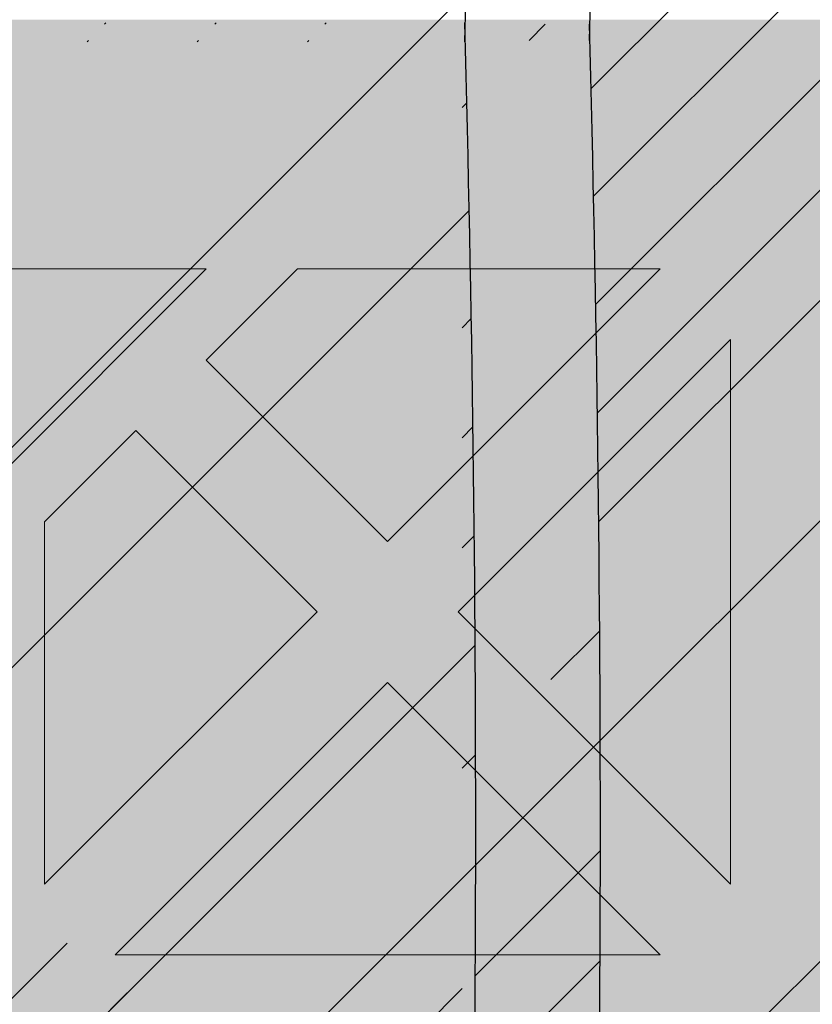
# Model space of a CAD drawing. Units: inches. Extents: x 844 to 2234, y 346 to 1084.
# Tile 11 of 93: x 1122.921 to 1124.948, y 693.702 to 696.22. Entities that reach past the tile are written whole.
import ezdxf

# ---------------------------------------------------------------- set-up
doc = ezdxf.new("R2010")
doc.units = ezdxf.units.IN
doc.header["$MEASUREMENT"] = 0
for name, color, linetype, lineweight in [('A-ANNO-DIMS', 2, 'Continuous', 18), ('furniture', 8, 'Continuous', 18), ('RA-AP-01$0$INT', 35, 'Continuous', 5)]:
    doc.layers.add(name, color=color, linetype=linetype, lineweight=lineweight)
doc.layers.add('RA-AP-01$0$FURN', color=3, linetype='Continuous')
doc.layers.add('RA-AP-01$0$WOOD', color=64, linetype='Continuous')
doc.styles.get("Standard").update_dxf_attribs({"font": 'arial.ttf'})
doc.dimstyles.get("Standard").update_dxf_attribs({"dimtxt": 6, "dimasz": 3, "dimexe": 0.18, "dimexo": 0.0625, "dimgap": 0.09, "dimtad": 0, "dimtih": 1, "dimtoh": 1, "dimdec": 1, "dimzin": 0, "dimdsep": 46, "dimlunit": 3, "dimtxsty": 'Standard', "dimblk": 'ARCHTICK', "dimcen": 0.09, "dimadec": 0, "dimazin": 0, "dimtfac": 1, "dimtdec": 1, "dimtofl": 0, "dimtmove": 0, "dimatfit": 3, "dimfxl": 1, "dimtolj": 1, "dimtzin": 0, "dimarcsym": 0})

# ---------------------------------------------------------------- blocks, each defined once
blk = doc.blocks.new('A$C18D01794')
at = {"layer": 'RA-AP-01$0$INT'}
h = blk.add_hatch(color=256, dxfattribs=at)
h.paths.add_polyline_path([(4.585917135068448, -6.356712009588273), (4.614201406330596, -6.356712009589021), (4.668846067270487, -6.411356670531338), (4.723490728212344, -6.356712009591912), (4.771774999457151, -6.35671200959319), (4.826419660396886, -6.411356670535356), (4.862780050090322, -6.374996280843536), (4.844495778842715, -6.356712009595112), (4.862780050090411, -6.356712009595595), (4.905206456960182, -6.399138416468211), (4.947632863832445, -6.356712009597838), (4.965917135079675, -6.356712009598322), (4.947632863831759, -6.374996280845421), (4.983993253523576, -6.411356670538857), (5.038637914464627, -6.356712009600247), (5.08692218571208, -6.356712009601523), (5.141566846649976, -6.411356670541852), (5.196211507589851, -6.356712009604411), (5.224495778822615, -6.356712009605161), (4.905206456953975, -6.676001331473793)])
h.paths.add_polyline_path([(4.895206456956031, -6.637717060225675), (4.895206456958921, -6.528427738347902), (4.840561796018589, -6.583072399285802)], flags=16)
h.paths.add_polyline_path([(4.915206456955638, -6.637717060226121), (4.969851117895509, -6.583072399288678), (4.915206456957609, -6.528427738348344)], flags=16)
h.paths.add_polyline_path([(4.826419660395175, -6.568930263661755), (4.881064321335613, -6.514285602723745), (4.771774999456703, -6.514285602720857)], flags=16)
h.paths.add_polyline_path([(4.983993253519558, -6.568930263665262), (5.038637914460456, -6.514285602726792), (4.929348592581548, -6.514285602724816)], flags=16)
h.paths.add_polyline_path([(4.881064321336025, -6.494285602723742), (4.826419660397532, -6.439640941782821), (4.771774999457062, -6.494285602720859)], flags=16)
h.paths.add_polyline_path([(4.929348592582019, -6.494285602724817), (5.038637914460982, -6.494285602726792), (4.983993253522945, -6.439640941786327)], flags=16)
h.paths.add_polyline_path([(4.895206456960191, -6.480143467100443), (4.895206456962115, -6.407422687715913), (4.876922185715016, -6.389138416467584), (4.840561796021581, -6.425498806159401)], flags=16)
h.paths.add_polyline_path([(4.915206456958487, -6.480143467100889), (4.969851117899527, -6.425498806162279), (4.933490728206909, -6.389138416468043), (4.9152064569598, -6.40742268771434)], flags=16)
h.paths.add_polyline_path([(4.757632863832376, -6.480143467096812), (4.812277524772842, -6.425498806158772), (4.757632863834348, -6.370854145217844)], flags=16)
h.paths.add_polyline_path([(4.737632863832376, -6.480143467096286), (4.737632863834348, -6.370854145217375), (4.682988202893906, -6.425498806155385)], flags=16)
h.paths.add_polyline_path([(5.05278005008503, -6.480143467103376), (5.052780050087917, -6.370854145224413), (4.998135389146995, -6.425498806162908)], flags=16)
h.paths.add_polyline_path([(5.072780050085024, -6.480143467103744), (5.127424711025931, -6.42549880616527), (5.072780050087916, -6.370854145224832)], flags=16)
h.paths.add_polyline_path([(4.935917135072783, -6.706712009592292), (5.255206456948811, -6.387422687716309), (5.255206456948932, -6.415706958964177), (5.200561796010279, -6.470351619902839), (5.255206456949403, -6.524996280841948), (5.25520645694961, -6.5732805520894), (5.200561796009787, -6.627925213029239), (5.236922185702417, -6.664285602721864), (5.255206456949919, -6.646001331474357), (5.255206456949998, -6.664285602721898), (5.212780050078687, -6.706712009592262), (5.25520645695036, -6.749138416463932), (5.255206456950438, -6.767422687711313), (5.236922185702424, -6.749138416463297), (5.200561796009796, -6.785498806155928), (5.255206456950753, -6.840143467096874), (5.25520645695096, -6.888427738341682), (5.200561796010322, -6.943072399282328), (5.255206456951428, -6.997717060223427), (5.255206456951547, -7.026001331471006)])
h.paths.add_polyline_path([(5.042988202883395, -6.785498806155427), (5.097632863823085, -6.840143467095101), (5.097632863822622, -6.730854145216193)], flags=16)
h.paths.add_polyline_path([(5.028846067259663, -6.771356670531693), (5.083490728198774, -6.716712009592573), (4.974201406321001, -6.716712009593042)], flags=16)
h.paths.add_polyline_path([(5.117632863823087, -6.840143467095186), (5.172277524762331, -6.785498806155926), (5.11763286382262, -6.730854145216225)], flags=16)
h.paths.add_polyline_path([(5.08349072819877, -6.696712009593886), (5.028846067259652, -6.642067348654775), (4.974201406320998, -6.696712009593438)], flags=16)
h.paths.add_polyline_path([(5.131774999446817, -6.854285602718917), (5.186419660386065, -6.799640941779662), (5.241064321325782, -6.854285602719365)], flags=17)
h.paths.add_polyline_path([(5.131774999446228, -6.716712009592374), (5.186419660386065, -6.771356670532194), (5.222780050079488, -6.734996280838764), (5.204495778832781, -6.716712009592063)], flags=16)
h.paths.add_polyline_path([(5.097632863822613, -6.682569873970264), (5.097632863823061, -6.573280552091354), (5.042988202883383, -6.627925213031044)], flags=16)
h.paths.add_polyline_path([(5.131774999446899, -6.874285602718915), (5.241064321325809, -6.874285602719364), (5.186419660386591, -6.928930263658598)], flags=17)
h.paths.add_polyline_path([(5.131774999446226, -6.696712009594078), (5.204495778830767, -6.696712009594374), (5.22278005007868, -6.67842773834687), (5.186419660386049, -6.642067348654249)], flags=16)
h.paths.add_polyline_path([(5.11763286382262, -6.682569873970225), (5.17227752476232, -6.627925213030515), (5.117632863823064, -6.573280552091267)], flags=16)
h.paths.add_polyline_path([(5.186419660386069, -6.613783077405491), (5.241064321325754, -6.559138416465795), (5.131774999446791, -6.559138416466263)], flags=16)
h.paths.add_polyline_path([(5.131774999446872, -6.539138416466263), (5.24106432132578, -6.539138416465794), (5.186419660386554, -6.484493755526573)], flags=16)
h.paths.add_polyline_path([(5.255206456951811, -7.08742268770861), (5.255206456951895, -7.106712009588038), (4.555206456956052, -7.106712009588038), (4.555206456956136, -7.087422687708617), (4.905206456953973, -6.737422687710788)])
h.paths.add_polyline_path([(4.983993253513404, -6.8444937555241), (4.92934859257295, -6.899138416462108), (5.03863791445186, -6.899138416465014)], flags=16)
h.paths.add_polyline_path([(4.969851117889988, -6.83035161990006), (4.915206456952556, -6.775706958960171), (4.915206456949648, -6.884996280837944)], flags=16)
h.paths.add_polyline_path([(4.929348592572535, -6.919138416462105), (4.983993253511019, -6.973783077403037), (5.038637914451496, -6.919138416465012)], flags=16)
h.paths.add_polyline_path([(5.052780050074912, -6.93328055208906), (4.998135389134438, -6.987925213027088), (5.052780050072919, -7.042569873968025)], flags=16)
h.paths.add_polyline_path([(5.07278005007491, -6.933280552089588), (5.072780050072918, -7.042569873968497), (5.127424711013374, -6.987925213030498)], flags=16)
h.paths.add_polyline_path([(4.89520645695295, -6.775706958959721), (4.840561796013067, -6.830351619897157), (4.895206456950961, -6.884996280837494)], flags=16)
h.paths.add_polyline_path([(4.915206456948365, -6.933280552085403), (4.915206456946434, -7.006001331471951), (4.933490728192729, -7.024285602719066), (4.969851117886972, -6.987925213026453)], flags=16)
h.paths.add_polyline_path([(4.881064321327021, -6.899138416461022), (4.82641966038902, -6.84449375552057), (4.771774999448108, -6.899138416459029)], flags=16)
h.paths.add_polyline_path([(4.895206456950073, -6.933280552084951), (4.840561796009022, -6.987925213023558), (4.876922185700835, -7.024285602716997), (4.895206456948749, -7.006001331469487)], flags=16)
h.paths.add_polyline_path([(4.983993253510392, -7.0020673486505), (4.947632863816944, -7.038427738342319), (4.965917135064043, -7.05671200959023), (5.038637914448995, -7.056712009591555)], flags=16)
h.paths.add_polyline_path([(4.881064321326543, -6.91913841646102), (4.771774999447578, -6.919138416459031), (4.826419660385607, -6.973783077399508)], flags=16)
h.paths.add_polyline_path([(4.905206456946447, -7.014285602717636), (4.862780050074785, -7.056712009588352), (4.947632863816685, -7.056712009589775)], flags=16)
h.paths.add_polyline_path([(5.14156684663679, -7.002067348654549), (5.086922185696452, -7.056712009592438), (5.196211507574223, -7.056712009594425)], flags=16)
h.paths.add_polyline_path([(4.8264196603837, -7.002067348646972), (4.771774999442643, -7.056712009585575), (4.8444957788276, -7.056712009587508), (4.862780050075511, -7.038427738340416)], flags=16)
h.paths.add_polyline_path([(4.812277524760289, -6.98792521302292), (4.757632863822258, -6.933280552082447), (4.757632863819352, -7.042569873961408)], flags=16)
h.paths.add_polyline_path([(4.73763286382226, -6.933280552082079), (4.682988202881349, -6.987925213020536), (4.737632863819352, -7.04256987396099)], flags=16)
h.paths.add_polyline_path([(4.723490728195188, -7.056712009584289), (4.668846067257299, -7.002067348643949), (4.614201406317417, -7.056712009581383)], flags=16)
h.paths.add_polyline_path([(4.597632863829262, -6.706712009592262), (4.555206456957951, -6.664285602721896), (4.555206456958029, -6.646001331474357), (4.573490728205535, -6.664285602721864), (4.609851117898167, -6.627925213029238), (4.555206456958338, -6.573280552089402), (4.555206456958546, -6.524996280841952), (4.60985111789767, -6.470351619902839), (4.555206456959015, -6.415706958964177), (4.555206456959138, -6.387422687716309), (4.874495778835167, -6.70671200959229), (4.5552064569564, -7.026001331471015), (4.555206456956523, -6.997717060223433), (4.609851117897629, -6.94307239928233), (4.555206456956988, -6.888427738341681), (4.555206456957198, -6.840143467096881), (4.609851117898153, -6.78549880615593), (4.573490728205528, -6.749138416463297), (4.555206456957507, -6.76742268771132), (4.555206456957585, -6.749138416463933)])
h.paths.add_polyline_path([(4.712780050085332, -6.730854145216195), (4.712780050084863, -6.840143467095105), (4.767424711024555, -6.785498806155427)], flags=16)
h.paths.add_polyline_path([(4.726922185709173, -6.716712009592573), (4.781566846648288, -6.771356670531693), (4.836211507586949, -6.716712009593043)], flags=16)
h.paths.add_polyline_path([(4.692780050085327, -6.730854145216225), (4.638135389145619, -6.785498806155928), (4.692780050084865, -6.840143467095185)], flags=16)
h.paths.add_polyline_path([(4.726922185709182, -6.696712009593886), (4.836211507586949, -6.696712009593436), (4.7815668466483, -6.642067348654773)], flags=16)
h.paths.add_polyline_path([(4.678637914461726, -6.71671200959237), (4.605917135075169, -6.716712009592063), (4.587632863828464, -6.734996280838766), (4.623993253521887, -6.771356670532195)], flags=16)
h.paths.add_polyline_path([(4.712780050085336, -6.68256987397026), (4.767424711024568, -6.627925213031042), (4.71278005008489, -6.573280552091352)], flags=16)
h.paths.add_polyline_path([(4.678637914461726, -6.696712009594076), (4.623993253521899, -6.642067348654247), (4.587632863829271, -6.67842773834687), (4.605917135077185, -6.696712009594376)], flags=16)
h.paths.add_polyline_path([(4.692780050085336, -6.682569873970228), (4.692780050084889, -6.573280552091267), (4.638135389145632, -6.627925213030515)], flags=16)
h.paths.add_polyline_path([(4.623993253521885, -6.799640941779662), (4.678637914461131, -6.854285602718915), (4.56934859258217, -6.854285602719365)], flags=17)
h.paths.add_polyline_path([(4.623993253521901, -6.613783077405509), (4.678637914461158, -6.559138416466263), (4.569348592582195, -6.559138416465795)], flags=16)
h.paths.add_polyline_path([(4.678637914461051, -6.874285602718915), (4.623993253521361, -6.928930263658598), (4.569348592582143, -6.874285602719364)], flags=17)
h.paths.add_polyline_path([(4.678637914461076, -6.539138416466263), (4.623993253521399, -6.484493755526573), (4.569348592582167, -6.539138416465796)], flags=16)
h = blk.add_hatch(color=256, dxfattribs=at)
h.paths.add_polyline_path([(4.895206456952951, -6.77570695895972), (4.840561796013068, -6.830351619897156), (4.895206456950958, -6.884996280837495)])
h.paths.add_polyline_path([(4.915206456949649, -6.884996280837942), (4.969851117889987, -6.830351619900054), (4.915206456952556, -6.775706958960171)])
h.paths.add_polyline_path([(5.038637914451862, -6.899138416465013), (4.983993253513403, -6.8444937555241), (4.929348592572953, -6.899138416462106)])
h.paths.add_polyline_path([(4.929348592572535, -6.919138416462105), (4.983993253511018, -6.973783077403037), (5.038637914451497, -6.919138416465012)])
h.paths.add_polyline_path([(4.915206456948366, -6.933280552085397), (4.915206456946433, -7.006001331471951), (4.93349072819273, -7.024285602719068), (4.969851117886972, -6.987925213026454)])
h.paths.add_polyline_path([(5.038637914448995, -7.056712009591553), (4.983993253510389, -7.002067348650502), (4.947632863816946, -7.038427738342318), (4.965917135064043, -7.05671200959023)])
h.paths.add_polyline_path([(5.05278005007292, -7.042569873968023), (5.05278005007491, -6.933280552089059), (4.998135389134438, -6.987925213027088)])
h.paths.add_polyline_path([(5.07278005007292, -7.042569873968496), (5.127424711013374, -6.987925213030498), (5.072780050074909, -6.933280552089588)])
h.paths.add_polyline_path([(5.141566846636789, -7.002067348654547), (5.086922185696449, -7.056712009592438), (5.196211507574223, -7.056712009594425)])
h.paths.add_polyline_path([(4.947632863816688, -7.056712009589774), (4.905206456946449, -7.014285602717634), (4.862780050074784, -7.056712009588353)])
h.paths.add_polyline_path([(4.840561796009025, -6.987925213023556), (4.876922185700834, -7.024285602716997), (4.895206456948747, -7.006001331469488), (4.895206456950075, -6.933280552084953)])
h.paths.add_polyline_path([(4.88106432132654, -6.919138416461021), (4.771774999447577, -6.919138416459031), (4.826419660385606, -6.973783077399508)])
h.paths.add_polyline_path([(4.881064321327019, -6.899138416461022), (4.826419660389019, -6.844493755520571), (4.771774999448108, -6.89913841645903)])
h.paths.add_polyline_path([(4.757632863819352, -7.042569873961409), (4.812277524760284, -6.987925213022922), (4.757632863822259, -6.933280552082447)])
h.paths.add_polyline_path([(4.8264196603837, -7.002067348646974), (4.771774999442646, -7.056712009585575), (4.844495778827599, -7.05671200958751), (4.862780050075512, -7.038427738340417)])
h.paths.add_polyline_path([(4.737632863819352, -7.042569873960988), (4.737632863822258, -6.933280552082078), (4.682988202881349, -6.987925213020538)])
h.paths.add_polyline_path([(4.668846067257299, -7.002067348643952), (4.61420140631742, -7.056712009581384), (4.723490728195189, -7.056712009584292)])
for p, q in [((5.038637914451498, -6.919138416465012), (4.929348592572535, -6.919138416462105)), ((4.929348592572535, -6.919138416462105), (4.983993253511019, -6.973783077403037)), ((5.038637914451498, -6.919138416465012), (4.983993253511019, -6.973783077403037)), ((4.915206456946434, -7.006001331470351), (4.915206456948367, -6.933280552085399)), ((4.915206456948367, -6.933280552085399), (4.969851117886972, -6.987925213026453)), ((5.05278005007491, -6.93328055208906), (4.998135389134438, -6.987925213027088)), ((5.05278005007491, -6.93328055208906), (5.052780050072921, -7.042569873968023)), ((4.969851117886972, -6.987925213026452), (4.93349072819353, -7.024285602718265)), ((5.052780050072921, -7.042569873968023), (4.998135389134438, -6.987925213027088)), ((4.98399325351039, -7.002067348650502), (4.947632863816946, -7.038427738342317)), ((5.038637914448995, -7.056712009591555), (4.983993253510388, -7.002067348650502)), ((4.915206456946427, -7.006001331471944), (4.933490728193524, -7.02428560271986)), ((4.905206456946449, -7.014285602717635), (4.94763286381669, -7.056712009589775)), ((4.947632863816946, -7.038427738342317), (4.965917135063997, -7.056712009590183)), ((4.965917135064043, -7.056712009590231), (4.947632863816944, -7.038427738342317)), ((4.94763286381669, -7.056712009589775), (4.862780050074783, -7.056712009588354)), ((4.965917135064043, -7.05671200959023), (5.038637914448995, -7.056712009591555))]:
    blk.add_line(p, q, dxfattribs=at)
blk = doc.blocks.new('A$C32926AE1')
at = {"layer": 'RA-AP-01$0$FURN'}
h = blk.add_hatch(dxfattribs=at)
h.set_pattern_fill('ANSI31', color=256, scale=0.1, style=0)
h.set_pattern_definition([(45, (0, 0), (-0.0088388347648318, 0.0088388347648318), [])])
edge = h.paths.add_edge_path(flags=16)
edge.add_arc((4.904771284329206, 4.246793130718756), 0.2603971832811541, 75.22398030683196, 104.7760196931204)
edge.add_arc((4.904771284329206, 4.246793130718756), 0.2603971832811541, 75.223980306832, 104.77601969312039, ccw=False)
edge = h.paths.add_edge_path(flags=16)
edge.add_arc((4.904771284329206, 4.067062675376612), 0.2603971832811541, 255.2239803068796, 284.776019693168)
edge.add_arc((4.904771284329206, 4.067062675376612), 0.2603971832811541, 255.22398030687958, 284.77601969316805, ccw=False)
edge = h.paths.add_edge_path(flags=0)
edge.add_arc((4.904771284329206, 4.067062675376612), 0.2603971832811541, 255.2239803068796, 284.776019693168)
edge.add_arc((4.904771284329206, 4.067062675376612), 0.2603971832811541, 255.22398030687958, 284.77601969316805, ccw=False)
edge = h.paths.add_edge_path(flags=0)
edge.add_arc((4.904771284329206, 4.067062675376612), 0.2603971832811541, 255.2239803068796, 284.776019693168)
edge.add_arc((4.904771284329206, 4.067062675376612), 0.2603971832811541, 255.22398030687958, 284.77601969316805, ccw=False)
edge = h.paths.add_edge_path()
edge.add_arc((4.604388392048174, 4.588829985554312), 0.1599999999999918, 342.3781640246255, 354.4317409793762)
edge.add_arc((5.090145208887507, 4.43216705527679), 0.3503971832811637, 162.0091218307731, 180.3186872093483)
edge.add_arc((5.205154176610243, 4.588829985554953), 0.1599999999999917, 185.5682590208461, 197.6218359767349)
edge.add_arc((4.904771284329229, 4.246793130718735), 0.3503971832811761, 72.00912183053516, 107.9908781690354)
edge.add_arc((9.535952835716557, 4.28682295566602), 4.798342501046485, 178.2875002453811, 181.5576802719453)
edge.add_arc((4.719397359771122, 4.43216705527679), 0.3503971832811637, 359.6813127906516, 377.9908781692269)
edge.add_arc((9.535967292294904, 4.286822350292874), 4.778371420254705, 178.2965938931842, 181.5667745797229)
edge.add_arc((4.719397359771122, 4.43216705527679), 0.3303971832811637, 359.6813127906516, 377.9908781692269)
edge.add_arc((0.2735752763637294, 4.286822350292874), 4.7783714202547, 358.4332254202771, 361.7034061068158)
edge.add_arc((5.061434214606998, 4.732549947558029), 0.1600000000000254, 252.3781640250584, 264.4317409792362)
edge.add_arc((4.748108354051257, 4.732549947558012), 0.1600000000000541, 275.5682590208426, 287.6218359759532)
edge.add_arc((4.604388392048115, 4.588829985554317), 0.1800000000000505, 342.3567572500182, 349.3735009646207)
edge.add_arc((5.205154176610254, 4.588829985554976), 0.1800000000000069, 190.6264990356027, 197.6432427513933)
edge.add_arc((5.061434214607106, 4.732549947558013), 0.1800000000000424, 252.3567572496606, 259.3735009644582)
edge.add_arc((4.904771284329208, 4.246793130718737), 0.3303971832811676, 71.99844483668534, 108.0015551637021)
edge.add_arc((4.748108354051414, 4.732549947558045), 0.1800000000000547, 280.6264990355479, 287.6432427495938)
edge.add_arc((5.090145208887514, 4.432167055276789), 0.2803971832811691, 162.8706300666893, 180.816523289902)
edge.add_arc((4.719397359771136, 4.432167055276689), 0.2803971832811534, 359.183476710103, 377.1293699333214)
edge.add_arc((4.904771284329222, 4.246793130718737), 0.2803971832811769, 72.87063006672916, 107.1293699332334)
edge.add_arc((5.090145208887522, 4.432167055276788), 0.2603971832811776, 165.2239803068007, 180.9953123810312)
edge.add_arc((4.719397359771141, 4.432167055276699), 0.2603971832811458, 359.0046876189768, 374.7760196932087)
edge.add_arc((5.090145208887507, 4.43216705527679), 0.3303971832811637, 162.0091218307731, 180.3186872093483)
edge.add_arc((9.53595427642584, 4.285015535491528), 4.728345371032053, 178.265043920078, 181.5679956281801)
edge.add_arc((0.2735882922327999, 4.285015535491582), 4.728345371032045, 358.4320043718193, 361.7349560799204)
edge.add_arc((9.535953591267507, 4.284458026472751), 4.708343996644348, 178.2573054306777, 181.5704995759608)
edge.add_arc((0.273588977391114, 4.284458026472785), 4.708343996644358, 358.4295004240388, 361.7426945693213)
edge.add_arc((0.2735889773911131, 4.029397779622582), 4.708343996644359, 358.2573054306787, 361.5704995759613)
edge.add_arc((9.535953591267518, 4.029397779622618), 4.708343996644359, 178.4295004240391, 181.7426945693223)
edge.add_arc((0.2735882922327901, 4.028840270603786), 4.728345371032054, 358.2650439200796, 361.5679956281808)
edge.add_arc((9.53595427642584, 4.028840270603841), 4.728345371032054, 178.4320043718199, 181.7349560799219)
edge.add_arc((0.2735752763637302, 4.027033455802493), 4.778371420254699, 358.2965938931842, 361.5667745797229)
edge.add_arc((4.719397359771122, 3.881688750818578), 0.3303971832811637, 342.0091218307731, 360.3186872093484)
edge.add_arc((5.090145208887507, 3.881688750818578), 0.3303971832811637, 179.6813127906516, 197.9908781692269)
edge.add_arc((9.535967292294904, 4.027033455802493), 4.778371420254705, 178.433225420277, 181.7034061068158)
edge.add_arc((4.719397359771122, 3.881688750818578), 0.3503971832811637, 342.0091218307731, 360.3186872093484)
edge.add_arc((9.53595283571655, 4.027032850429349), 4.79834250104648, 178.4423197280546, 181.7124997546188)
edge.add_arc((4.719397359771141, 3.881688750818669), 0.2603971832811458, 345.2239803067913, 360.9953123810232)
edge.add_arc((5.090145208887522, 3.88168875081858), 0.2603971832811776, 179.0046876189687, 194.7760196931993)
edge.add_arc((4.904771284329222, 4.067062675376631), 0.2803971832811769, 252.8706300667665, 287.1293699332708)
edge.add_arc((4.719397359771136, 3.881688750818678), 0.2803971832811534, 342.8706300666787, 360.8165232898969)
edge.add_arc((5.090145208887514, 3.881688750818579), 0.2803971832811691, 179.183476710098, 197.1293699333106)
edge.add_arc((4.748108354051414, 3.581305858537323), 0.1800000000000547, 72.3567572504062, 79.37350096445199)
edge.add_arc((4.904771284329208, 4.067062675376631), 0.3303971832811676, 251.9984448362979, 288.0015551633146)
edge.add_arc((5.061434214607106, 3.581305858537355), 0.1800000000000424, 100.6264990355418, 107.6432427503394)
edge.add_arc((5.205154176610254, 3.725025820540392), 0.1800000000000069, 162.3567572486066, 169.3735009643972)
edge.add_arc((4.604388392048115, 3.725025820541051), 0.1800000000000505, 10.62649903537925, 17.64324274998182)
edge.add_arc((4.748108354051257, 3.581305858537356), 0.1600000000000541, 72.37816402404681, 84.43174097915735)
edge.add_arc((4.904771284329229, 4.067062675376632), 0.3503971832811761, 252.0091218309645, 287.9908781694648)
edge.add_arc((5.061434214606998, 3.581305858537339), 0.1600000000000254, 95.56825902076373, 107.6218359749416)
edge.add_arc((5.205154176610243, 3.725025820540414), 0.1599999999999917, 162.3781640232651, 174.4317409791539)
edge.add_arc((5.090145208887507, 3.881688750818578), 0.3503971832811637, 179.6813127906516, 197.9908781692269)
edge.add_arc((4.604388392048174, 3.725025820541056), 0.1599999999999918, 5.568259020623824, 17.62183597537444)
edge.add_arc((0.2735897329420762, 4.28682295566602), 4.798342501046482, 358.4423197280547, 361.7124997546188)
edge.add_arc((0.2735897329420691, 4.027032850429348), 4.798342501046489, 358.2875002453812, 361.5576802719453)
at = {"layer": 'RA-AP-01$0$WOOD'}
h = blk.add_hatch(color=256, dxfattribs=at)
h.dxf.hatch_style = 1
h.paths.add_polyline_path([(5.157430609644524, 4.573483066760929, -0.1009492694046607), (5.155401577623758, 4.593365984175333, -0.1842662638101597), (5.172249623284174, 4.638795604568598, 0.2056608120311276), (5.179560981299304, 4.661316324430096, 0.3614336704623542), (5.134352340494423, 4.706524965234944, 0.2056608120311297), (5.111831620632933, 4.699213607219793, -0.1842662638101113), (5.066402000239693, 4.682365561559342, -0.1055311479399994), (5.045656153913092, 4.68467289944697, 0.1567636581983829), (4.763886414745334, 4.684672899446966, -0.1055311479399895), (4.743140568418733, 4.68236556155934, -0.1842662638100833), (4.6977109480255, 4.69921360721979, 0.2056608120302612), (4.675190228164109, 4.706524965234949, 0.3614336704708441), (4.629981587358889, 4.66131632442871, 0.2056608120245944), (4.637292945374126, 4.638795604567974, -0.1842662638101024), (4.654140991034615, 4.59336598417475, -0.1009492694055169), (4.652111959013835, 4.573483066760181, 0.021410119221476), (4.629748025606143, 4.156712009541676, 0.0214101192214795), (4.652111959013809, 3.739940952323101, -0.1009492694059586), (4.654140991034615, 3.720058034908448, -0.1842662638100975), (4.637292945374126, 3.674628414515226, 0.2056608120245705), (4.629981587358889, 3.652107694654492, 0.3614336704708879), (4.675190228164113, 3.606899053848249, 0.2056608120302384), (4.697710948025501, 3.614210411863408, -0.1842662638100995), (4.743140568418738, 3.63105845752386, -0.1055311479402541), (4.763886414745388, 3.628751119636215, 0.1567636581983776), (5.045656153913137, 3.628751119636244, -0.1055311479397538), (5.066402000239692, 3.631058457523857, -0.1842662638101067), (5.111831620632931, 3.614210411863407, 0.2056608120310924), (5.134352340494417, 3.606899053848256, 0.3614336704624001), (5.179560981299307, 3.652107694653103, 0.2056608120311314), (5.172249623284175, 3.6746284145146, -0.1842662638101402), (5.155401577623758, 3.72005803490786, -0.1009492694051366), (5.15743060964455, 3.739940952322354, 0.0214101192215073), (5.179794543052287, 4.156712009541468, 0.0214101192215252)])
h.paths.add_polyline_path([(4.639748609479751, 4.156712009541513, 0.0213537860821624), (4.661970494867118, 3.741887061152232, -0.094075836301374), (4.664143710413708, 3.7196126951003, -0.1824818158568985), (4.644813765429836, 3.668037719127816, 0.2056608120245319), (4.639939526753007, 3.653023905887301, 0.3614336704710246), (4.676106439397173, 3.616856993242342, 0.2056608120302234), (4.691120252638095, 3.621731231919122, -0.1824818158602558), (4.742695228611606, 3.641061176902986, -0.1029891339458722), (4.766991894714349, 3.638256818950944, 0.156709409989566), (5.042550673941472, 3.638256818950105, -0.102989133958497), (5.066847340047078, 3.641061176902949, -0.1824818158594995), (5.118422316020358, 3.621731231919103, 0.2056608120311416), (5.133436129261316, 3.616856993242346, 0.3614336704621468), (5.169603041905217, 3.653023905886178, 0.2056608120310986), (5.164728803228477, 3.668037719127177, -0.1824818158565612), (5.145398858244737, 3.719612695099578, -0.0940758363009313), (5.147572073791232, 3.741887061151398, 0.0213537860822023), (5.169793959178681, 4.156712009541451, 0.0213537860822226), (5.147572073791203, 4.571536957931898, -0.0940758363005034), (5.145398858244737, 4.59381132398362, -0.1824818158565587), (5.164728803228476, 4.645386299956021, 0.2056608120311045), (5.169603041905216, 4.66040011319702, 0.3614336704621845), (5.133436129261313, 4.696567025840856, 0.2056608120310773), (5.118422316020359, 4.691692787164098, -0.182481815859508), (5.066847340047078, 4.67236284218025, -0.1029891339584606), (5.04255067394148, 4.675167200133092, 0.156709409989566), (4.766991894714357, 4.675167200132257, -0.1029891339458842), (4.742695228611611, 4.672362842180213, -0.1824818158602725), (4.691120252638095, 4.691692787164077, 0.2056608120302152), (4.676106439397174, 4.696567025840858, 0.3614336704710363), (4.639939526753005, 4.660400113195899, 0.2056608120245495), (4.644813765429837, 4.645386299955384, -0.1824818158568934), (4.664143710413708, 4.593811323982902, -0.0940758363009187), (4.661970494867149, 4.571536957931074, 0.021353786082177)], flags=16)
h.paths.add_polyline_path([(5.129794543052235, 4.432167055276933, -0.0141661062790638), (5.130152669293814, 4.156927903047693, -0.0141661062790647), (5.129794543052234, 3.881688750818433, -0.0785247771143638), (5.10979738006795, 3.755143611847103, 0.0945969212073497), (5.105408519571111, 3.717898134952927, 0.1043170707844957), (5.116074640131521, 3.670385395016088, 0.1043170707864965), (5.068561900193738, 3.681051515576561, 0.09459692119553), (5.031316423304057, 3.676662655080835, -0.1580239521427272), (4.778226145355827, 3.676662655080367, 0.0945969211986668), (4.740980668464973, 3.681051515576592, 0.1043170707882822), (4.693467928526415, 3.670385395015844, 0.1043170707867916), (4.704134049087309, 3.717898134953662, 0.0945969211972894), (4.69974518859162, 3.755143611844042, -0.0785247771163196), (4.679748025606343, 3.881688750818406, -0.0141661062790663), (4.679389899364763, 4.156927903047693, -0.0141661062790672), (4.679748025606343, 4.432167055276998, -0.0785247771163064), (4.699745188591625, 4.55871219425134, 0.094596921197333), (4.704134049087308, 4.595957671141738, 0.1043170707867205), (4.693467928526416, 4.643470411079523, 0.1043170707882628), (4.740980668464965, 4.632804290518776, 0.0945969211988114), (4.778226145355874, 4.637193151015016, -0.158023952142669), (5.031316423304015, 4.637193151014546, 0.0945969211956361), (5.068561900193736, 4.632804290518806, 0.1043170707864979), (5.11607464013152, 4.643470411079278, 0.1043170707844617), (5.105408519571112, 4.595957671142455, 0.0945969212074597), (5.109797380067959, 4.558712194248236, -0.0785247771143467)], flags=0)
h.paths.add_polyline_path([(5.119794532311105, 4.432259799204851, -0.0142000800617244), (5.120156169157484, 4.156927903047701, -0.0142000800617277), (5.119794532311105, 3.881596006890482, -0.0784894509520253), (5.100273383573699, 3.758192358677797, 0.0940138827242913), (5.095413455884425, 3.717477693979438, 0.0606271852308753), (5.099615656341024, 3.686844378806616, 0.0606271852322524), (5.068982341167493, 3.691046579263239, 0.0940138827010453), (5.028267676478798, 3.686186651576848, -0.1580706864508061), (4.781274892180912, 3.686186651576435, 0.0940138827026903), (4.740560227491556, 3.691046579263279, 0.0606271852339895), (4.709926912317155, 3.686844378806508, 0.0606271852329405), (4.714129112773991, 3.717477693980356, 0.094013882701304), (4.709269185087677, 3.758192358669163, -0.0784894509577193), (4.689748036347473, 3.881596006890469, -0.014200080061729), (4.689386399501094, 4.156927903047709, -0.0142000800617217), (4.689748036347473, 4.432259799204808, -0.078489450957724), (4.709269185087651, 4.555663447426125, 0.0940138827014585), (4.714129112773992, 4.596378112114996, 0.0606271852329731), (4.709926912317154, 4.62701142728886, 0.0606271852340196), (4.74056022749157, 4.622809226832087, 0.0940138827024997), (4.781274892180847, 4.627669154518912, -0.1580706864508359), (5.028267676478777, 4.627669154518526, 0.0940138827010946), (5.068982341167492, 4.622809226832129, 0.060627185232254), (5.099615656341024, 4.627011427288751, 0.0606271852308727), (5.095413455884425, 4.59637811211593, 0.0940138827241088), (5.100273383573675, 4.555663447417647, -0.0784894509520978)], flags=0)
h.paths.add_polyline_path([(5.06978912287499, 4.430218106756144, -0.014241683694547), (5.070173729147532, 4.156927903047672, -0.0142416836945458), (5.06978912287499, 3.883637699339223, -0.0800609523125196), (5.052662118612511, 3.773463122773442, 0.0526421978001116), (5.04590916754064, 3.740550867606997, 0.0526421977992423), (5.012996912374707, 3.73379791653534, -0.1583028414718258), (4.796545656286308, 3.73379791653451, 0.0526421978034211), (4.763633401117837, 3.740550867607021, 0.0526421978018622), (4.756880450045755, 3.773463122774558, -0.0800609523117106), (4.739753445783639, 3.883637699339268, -0.0142416836945435), (4.739368839511098, 4.156927903047671, -0.0142416836945477), (4.739753445783639, 4.430218106756155, -0.0800609523116345), (4.75688045004574, 4.540392683320762, 0.052642197801941), (4.763633401117837, 4.573304938488346, 0.0526421978035071), (4.796545656286361, 4.580057889560873, -0.1583028414717561), (5.012996912374669, 4.580057889560039, 0.0526421977993048), (5.04590916754064, 4.57330493848837, 0.0526421978002057), (5.052662118612529, 4.540392683321868, -0.080060952312477)], flags=0)
h.paths.add_polyline_path([(5.049789715110557, 4.43038092723357, -0.0143097550741839), (5.05018085590259, 4.156927903047715, -0.0143097550741854), (5.049789715110558, 3.883474878861827, -0.0800685599149176), (5.03362098255317, 3.779581877367999, 0.0306258898956367), (5.028241146483733, 3.758218888663947, 0.0306258898977031), (5.006878157778253, 3.75283905259408, -0.1583983521624096), (4.802664410878162, 3.752839052594731, 0.0306258898946014), (4.781301422174808, 3.758218888663924, 0.0306258898967912), (4.775921586105202, 3.779581877368794, -0.080068559914251), (4.759752853548071, 3.883474878861786, -0.0143097550741854), (4.759361712756037, 4.156927903047671, -0.0143097550741854), (4.759752853548071, 4.430380927233557, -0.0800685599142479), (4.775921586105193, 4.534273928726546, 0.0306258898968306), (4.781301422174808, 4.555636917431444, 0.0306258898945754), (4.802664410878143, 4.561016753500631, -0.1583983521624168), (5.006878157778244, 4.561016753501291, 0.0306258898977177), (5.028241146483733, 4.555636917431421, 0.0306258898958182), (5.03362098255321, 4.534273928727244, -0.080068559914796)], flags=0)
h.paths.add_polyline_path([(4.999766070382627, 4.428171244713864, -0.0143443147609634), (5.000198441819402, 4.156927903047689, -0.0143443147609612), (4.999766070382627, 3.885684561381556, -0.0784641635803329), (4.987356730658798, 3.799103304488872, -0.1506053783831347), (4.822185837999821, 3.79910330448882, -0.0784641635803318), (4.809776498276007, 3.885684561381509, -0.014344314760963), (4.809344126839227, 4.156927903047677, -0.0143443147609645), (4.809776498276007, 4.428171244713873, -0.0784641635803192), (4.822185837999822, 4.514752501606549, -0.1506053783831338), (4.987356730658798, 4.514752501606494, -0.078464163580285)], flags=0)
h.paths.add_polyline_path([(4.979755254238824, 4.42764379880488, -0.0143772539198268), (4.980205517789977, 4.156927903047693, -0.0143772539198275), (4.979755254238824, 3.886212007290489, -0.0689242507424422), (4.971183264704897, 3.815276770442801, -0.1296645318904179), (4.838359303953726, 3.815276770442746, -0.0689242507424186), (4.829787314419809, 3.886212007290419, -0.0143772539198292), (4.829337050868653, 4.156927903047653, -0.0143772539198325), (4.829787314419809, 4.427643798804946, -0.0689242507424211), (4.838359303953725, 4.498579035652621, -0.1296645318904187), (4.971183264704897, 4.498579035652565, -0.0689242507424401)], flags=0)
h = blk.add_hatch(color=256, dxfattribs=at)
h.dxf.hatch_style = 1
h.paths.add_polyline_path([(5.145398858244737, 4.59381132398362, -0.1824818158565616), (5.164728803228476, 4.645386299956021, 0.2056608120311045), (5.169603041905216, 4.66040011319702, 0.3614336704621845), (5.133436129261313, 4.696567025840856, 0.2056608120310773), (5.118422316020359, 4.691692787164098, -0.182481815859508), (5.066847340047078, 4.67236284218025, -0.1029891339584606), (5.04255067394148, 4.675167200133092, 0.156709409989566), (4.766991894714357, 4.675167200132257, -0.1029891339458842), (4.742695228611611, 4.672362842180213, -0.1824818158602725), (4.691120252638095, 4.691692787164077, 0.2056608120302152), (4.676106439397174, 4.696567025840858, 0.3614336704710363), (4.639939526753005, 4.660400113195899, 0.2056608120245495), (4.644813765429837, 4.645386299955384, -0.1824818158568934), (4.664143710413708, 4.593811323982902, -0.0940758363009187), (4.661970494867149, 4.571536957931074, 0.0213537860821772), (4.639748609479751, 4.156712009541507, 0.0213537860821625), (4.661970494867119, 3.741887061152226, -0.0940758363013071), (4.664143710413708, 3.719612695100309, -0.1824818158569294), (4.644813765429836, 3.668037719127816, 0.2056608120245319), (4.639939526753007, 3.653023905887301, 0.3614336704710246), (4.676106439397173, 3.616856993242342, 0.2056608120302234), (4.691120252638095, 3.621731231919122, -0.1824818158602558), (4.742695228611606, 3.641061176902986, -0.1029891339458722), (4.766991894714349, 3.638256818950944, 0.156709409989566), (5.042550673941472, 3.638256818950105, -0.102989133958497), (5.066847340047078, 3.641061176902949, -0.1824818158594995), (5.118422316020358, 3.621731231919103, 0.2056608120311416), (5.133436129261316, 3.616856993242346, 0.3614336704621468), (5.169603041905217, 3.653023905886178, 0.2056608120310986), (5.164728803228477, 3.668037719127177, -0.1824818158565612), (5.145398858244737, 3.719612695099578, -0.0940758363009313), (5.147572073791232, 3.741887061151398, 0.0213537860822023), (5.169793959178681, 4.156712009541451, 0.0213537860822226), (5.147572073791203, 4.571536957931898, -0.0940758363004996)])
h.paths.add_polyline_path([(5.109797380067958, 4.55871219424824, -0.0785247771143472), (5.129794543052234, 4.432167055276936, -0.0141661062790644), (5.130152669293814, 4.156927903047685, -0.014166106279066), (5.129794543052234, 3.881688750818401, -0.0785247771143517), (5.109797380067946, 3.755143611847092, 0.0945969212073132), (5.105408519571111, 3.717898134952929, 0.1043170707844995), (5.116074640131521, 3.670385395016088, 0.1043170707864965), (5.068561900193738, 3.681051515576561, 0.09459692119553), (5.031316423304057, 3.676662655080835, -0.1580239521427272), (4.778226145355827, 3.676662655080367, 0.0945969211986668), (4.740980668464973, 3.681051515576592, 0.1043170707882822), (4.693467928526415, 3.670385395015844, 0.1043170707867916), (4.704134049087309, 3.717898134953662, 0.0945969211972894), (4.69974518859162, 3.755143611844042, -0.0785247771163196), (4.679748025606343, 3.881688750818406, -0.0141661062790663), (4.679389899364763, 4.156927903047693, -0.0141661062790672), (4.679748025606343, 4.432167055276998, -0.0785247771163064), (4.699745188591625, 4.55871219425134, 0.094596921197333), (4.704134049087308, 4.595957671141738, 0.1043170707867205), (4.693467928526416, 4.643470411079523, 0.1043170707882628), (4.740980668464965, 4.632804290518776, 0.0945969211988114), (4.778226145355874, 4.637193151015016, -0.158023952142669), (5.031316423304015, 4.637193151014546, 0.0945969211956361), (5.068561900193736, 4.632804290518806, 0.1043170707864979), (5.11607464013152, 4.643470411079278, 0.1043170707844617), (5.105408519571112, 4.595957671142455, 0.0945969212074504)], flags=16)
h.paths.add_polyline_path([(5.100273383573655, 4.55566344741771, -0.0784894509521388), (5.119794532311105, 4.432259799204852, -0.0142000800617252), (5.120156169157484, 4.156927903047686, -0.014200080061726), (5.119794532311105, 3.881596006890502, -0.0784894509520446), (5.100273383573696, 3.758192358677786, 0.0940138827242721), (5.095413455884425, 3.717477693979436, 0.0606271852308692), (5.099615656341024, 3.686844378806616, 0.0606271852322522), (5.068982341167493, 3.691046579263239, 0.0940138827010453), (5.028267676478798, 3.686186651576848, -0.1580706864508061), (4.781274892180912, 3.686186651576435, 0.0940138827026903), (4.740560227491556, 3.691046579263279, 0.0606271852339895), (4.709926912317155, 3.686844378806508, 0.0606271852329405), (4.714129112773991, 3.717477693980356, 0.094013882701304), (4.709269185087677, 3.758192358669163, -0.0784894509577193), (4.689748036347473, 3.881596006890469, -0.014200080061729), (4.689386399501094, 4.156927903047709, -0.0142000800617217), (4.689748036347473, 4.432259799204808, -0.078489450957724), (4.709269185087651, 4.555663447426125, 0.0940138827014585), (4.714129112773992, 4.596378112114996, 0.0606271852329731), (4.709926912317154, 4.62701142728886, 0.0606271852340196), (4.74056022749157, 4.622809226832087, 0.0940138827024997), (4.781274892180847, 4.627669154518912, -0.1580706864508359), (5.028267676478777, 4.627669154518526, 0.0940138827010946), (5.068982341167492, 4.622809226832129, 0.060627185232254), (5.099615656341024, 4.627011427288751, 0.0606271852308727), (5.095413455884425, 4.59637811211593, 0.094013882723957)], flags=0)
h.paths.add_polyline_path([(5.04590916754064, 4.57330493848837, 0.0526421978002057), (5.052662118612529, 4.540392683321868, -0.0800609523124783), (5.06978912287499, 4.430218106756142, -0.0142416836945469), (5.070173729147532, 4.156927903047672, -0.0142416836945458), (5.06978912287499, 3.883637699339223, -0.0800609523125196), (5.052662118612511, 3.773463122773442, 0.0526421978001116), (5.04590916754064, 3.740550867606997, 0.0526421977992423), (5.012996912374707, 3.73379791653534, -0.1583028414718258), (4.796545656286308, 3.73379791653451, 0.0526421978034211), (4.763633401117837, 3.740550867607021, 0.0526421978018622), (4.756880450045755, 3.773463122774558, -0.0800609523117106), (4.739753445783639, 3.883637699339268, -0.0142416836945435), (4.739368839511098, 4.156927903047671, -0.0142416836945477), (4.739753445783639, 4.430218106756155, -0.0800609523116345), (4.75688045004574, 4.540392683320762, 0.052642197801941), (4.763633401117837, 4.573304938488346, 0.0526421978035071), (4.796545656286361, 4.580057889560873, -0.1583028414717561), (5.012996912374669, 4.580057889560039, 0.0526421977993048)], flags=0)
h.paths.add_polyline_path([(5.028241146483733, 4.555636917431422, 0.0306258898956949), (5.033620982553182, 4.534273928727329, -0.0800685599148649), (5.049789715110557, 4.430380927233569, -0.0143097550741839), (5.05018085590259, 4.156927903047715, -0.0143097550741854), (5.049789715110558, 3.883474878861827, -0.0800685599149176), (5.03362098255317, 3.779581877367999, 0.0306258898956367), (5.028241146483733, 3.758218888663947, 0.0306258898977031), (5.006878157778253, 3.75283905259408, -0.1583983521624096), (4.802664410878162, 3.752839052594731, 0.0306258898946014), (4.781301422174808, 3.758218888663924, 0.0306258898967912), (4.775921586105202, 3.779581877368794, -0.080068559914251), (4.759752853548071, 3.883474878861786, -0.0143097550741854), (4.759361712756037, 4.156927903047671, -0.0143097550741854), (4.759752853548071, 4.430380927233557, -0.0800685599142479), (4.775921586105193, 4.534273928726546, 0.0306258898968306), (4.781301422174808, 4.555636917431444, 0.0306258898945754), (4.802664410878143, 4.561016753500631, -0.1583983521624168), (5.006878157778244, 4.561016753501291, 0.0306258898977174)], flags=0)
h.paths.add_polyline_path([(4.987356730658798, 4.514752501606494, -0.0784641635803018), (4.999766070382627, 4.428171244713845, -0.0143443147609637), (5.000198441819402, 4.156927903047665, -0.0143443147609622), (4.999766070382628, 3.885684561381514, -0.0784641635802952), (4.987356730658797, 3.799103304488872, -0.1506053783831338), (4.822185837999821, 3.799103304488819, -0.0784641635803342), (4.809776498276007, 3.885684561381512, -0.0143443147609628), (4.809344126839227, 4.156927903047676, -0.0143443147609646), (4.809776498276007, 4.428171244713873, -0.0784641635803192), (4.822185837999822, 4.514752501606549, -0.1506053783831338)], flags=0)
h.paths.add_polyline_path([(4.971183264704897, 4.498579035652566, -0.0689242507424384), (4.979755254238824, 4.427643798804883, -0.0143772539198276), (4.980205517789977, 4.15692790304768, -0.0143772539198258), (4.979755254238823, 3.88621200729051, -0.0689242507424628), (4.971183264704897, 3.815276770442801, -0.129664531890417), (4.838359303953726, 3.815276770442746, -0.0689242507424186), (4.829787314419809, 3.886212007290419, -0.0143772539198292), (4.829337050868653, 4.156927903047653, -0.0143772539198325), (4.829787314419809, 4.427643798804946, -0.0689242507424211), (4.838359303953725, 4.498579035652621, -0.1296645318904187)], flags=0)
h = blk.add_hatch(dxfattribs=at)
h.set_pattern_fill('ANSI31', color=256, scale=0.05, style=0)
h.set_pattern_definition([(45, (0, 0), (-0.0044194173824159, 0.0044194173824159), [])])
h.paths.add_polyline_path([(5.130152669293814, 4.156927903047704, 0.0141661062790657), (5.129794543052234, 4.432167055276982, 0.0777827904001433), (5.110168979996553, 4.557559993161921, -0.0976515123401879), (5.105408519571111, 4.595957671142454, -0.1043170707844687), (5.116074640131522, 4.64347041107928), (5.099615656341024, 4.627011427288751, 0.0606271852308727), (5.095413455884425, 4.59637811211593, 0.0940138827241088), (5.100273383573675, 4.555663447417647, -0.0784894509520972), (5.119794532311105, 4.432259799204852, -0.0142000800617252), (5.120156169157484, 4.156927903047686, -0.014200080061726), (5.119794532311105, 3.881596006890502, -0.0784894509520446), (5.100273383573696, 3.758192358677786, 0.0940138827242721), (5.095413455884425, 3.717477693979436, 0.0606271852308692), (5.099615656341024, 3.686844378806616), (5.116074640131519, 3.67038539501609, -0.1043170707844594), (5.105408519571112, 3.717898134952912, -0.0976515123401594), (5.11016897999655, 3.756295812933435, 0.0777827904001654), (5.129794543052234, 3.881688750818409, 0.0141661062790665)])
h.paths.add_polyline_path([(5.030164222210597, 3.676291055149937, -0.0976515123472002), (5.068561900193739, 3.681051515576561, -0.1043170707864927), (5.116074640131521, 3.670385395016088), (5.099615656341024, 3.686844378806616, 0.0606271852322522), (5.068982341167493, 3.691046579263239, 0.0940138827010453), (5.028267676478798, 3.686186651576848, -0.1580706864508061), (4.781274892180912, 3.686186651576435, 0.0940138827026903), (4.740560227491556, 3.691046579263279, 0.0606271852339913), (4.709926912317154, 3.686844378806508), (4.693467928526416, 3.670385395015845, -0.1043170707882796), (4.740980668464973, 3.681051515576592, -0.0976515123427246), (4.779378346446416, 3.676291055150394, 0.156512506893803)])
h.paths.add_polyline_path([(4.689748036347473, 3.881596006890472, -0.014200080061729), (4.689386399501094, 4.156927903047712, -0.0142000800617195), (4.689748036347473, 4.432259799204768, -0.078489450957742), (4.709269185087648, 4.555663447426114, 0.0940138827014821), (4.714129112773992, 4.596378112114995, 0.0606271852329748), (4.709926912317154, 4.62701142728886), (4.693467928526414, 4.643470411079524, -0.1043170707867939), (4.704134049087309, 4.595957671141706, -0.09765151234893), (4.699373588660725, 4.557559993157876, 0.0777827903975372), (4.679748025606343, 4.432167055276987, 0.0141661062790675), (4.679389899364763, 4.156927903047675, 0.0141661062790641), (4.679748025606343, 3.88168875081843, 0.0777827903975637), (4.699373588660724, 3.756295812937497, -0.0976515123490278), (4.704134049087308, 3.717898134953629, -0.1043170707867196), (4.693467928526416, 3.670385395015845), (4.709926912317155, 3.686844378806508, 0.0606271852329413), (4.714129112773991, 3.717477693980357, 0.0940138827013084), (4.709269185087676, 3.758192358669166, -0.0784894509577192)])
h.paths.add_polyline_path([(4.779378346446434, 4.63756475094498, -0.0976515123427943), (4.740980668464964, 4.632804290518776, -0.1043170707882609), (4.693467928526416, 4.643470411079523), (4.709926912317154, 4.62701142728886, 0.0606271852340196), (4.74056022749157, 4.622809226832087, 0.0940138827024997), (4.781274892180847, 4.627669154518912, -0.1580706864508359), (5.028267676478777, 4.627669154518526, 0.0940138827010946), (5.068982341167492, 4.622809226832129, 0.060627185232254), (5.099615656341024, 4.627011427288751), (5.116074640131521, 4.643470411079279, -0.1043170707865022), (5.068561900193735, 4.632804290518806, -0.0976515123475899), (5.030164222210446, 4.637564750945479, 0.1565125068936924)])
h = blk.add_hatch(dxfattribs=at)
h.set_pattern_fill('ANSI32', color=256, scale=0.2, style=0)
h.set_pattern_definition([(45, (0, 0), (-0.0530330085889911, 0.0530330085889911), []), (45, (0.035355339, 0), (-0.0530330085889911, 0.0530330085889911), [])])
h.paths.add_polyline_path([(5.119794532311105, 4.432259799204823, 0.0777015974868765), (5.10065834347252, 4.554469821747928, -0.0968902511992216), (5.095413455884425, 4.596378112115931, -0.060627185230871), (5.099615656341024, 4.627011427288751, -0.060627185232254), (5.068982341167492, 4.622809226832129, -0.0968902512198245), (5.027074050790956, 4.628054114423209, 0.1564657949319105), (4.782468517866163, 4.628054114422785, -0.0968902512152247), (4.740560227491555, 4.622809226832088, -0.0606271852339878), (4.709926912317155, 4.627011427288859, -0.0606271852329413), (4.714129112773991, 4.596378112115011, -0.0968902512205338), (4.708884225182929, 4.554469821738175, 0.0777015974804443), (4.689748036347473, 4.43225979920482, 0.0142000800617215), (4.689386399501094, 4.156927903047726, 0.0142000800617273), (4.689748036347473, 3.88159600689052, 0.077701597480541), (4.708884225182985, 3.759385984357019, -0.096890251220082), (4.714129112773992, 3.717477693980371, -0.0606271852329731), (4.709926912317154, 3.686844378806507, -0.060627185233988), (4.740560227491554, 3.691046579263279, -0.0968902512152569), (4.782468517866175, 3.685801691672578, 0.1564657949319236), (5.027074050790988, 3.685801691672169, -0.0968902512197451), (5.068982341167491, 3.691046579263239, -0.0606271852322557), (5.099615656341024, 3.686844378806616, -0.0606271852308727), (5.095413455884425, 3.717477693979438, -0.0968902511991229), (5.100658343472507, 3.7593859843474, 0.0777015974868745), (5.119794532311105, 3.8815960068905, 0.014200080061726), (5.120156169157484, 4.156927903047685, 0.0142000800617238)])
h.paths.add_polyline_path([(5.070173729147531, 4.156927903047684, -0.0142416836945481), (5.06978912287499, 3.883637699339191, -0.0800609523125107), (5.052662118612505, 3.773463122773424, 0.0526421978000811), (5.04590916754064, 3.740550867606997, 0.0526421977993214), (5.012996912374658, 3.733797916535325, -0.1583028414717916), (4.796545656286304, 3.733797916534512, 0.0526421978034138), (4.763633401117837, 3.740550867607021, 0.0526421978018622), (4.756880450045755, 3.773463122774558, -0.0800609523117106), (4.739753445783639, 3.883637699339268, -0.0142416836945435), (4.739368839511098, 4.156927903047671, -0.0142416836945477), (4.739753445783639, 4.430218106756155, -0.0800609523116345), (4.75688045004574, 4.540392683320762, 0.052642197801941), (4.763633401117837, 4.573304938488346, 0.0526421978035071), (4.796545656286361, 4.580057889560873, -0.1583028414717561), (5.012996912374669, 4.580057889560039, 0.0526421977993048), (5.04590916754064, 4.57330493848837, 0.0526421978002057), (5.052662118612529, 4.540392683321868, -0.0800609523124783), (5.06978912287499, 4.430218106756142, -0.0142416836945463)], flags=16)
h.paths.add_polyline_path([(5.050180855902591, 4.156927903047686, -0.0143097550741856), (5.049789715110558, 3.883474878861795, -0.0800685599148126), (5.033620982553202, 3.7795818773681, 0.0306258898957837), (5.028241146483733, 3.758218888663947, 0.0306258898977031), (5.006878157778253, 3.75283905259408, -0.1583983521624096), (4.802664410878162, 3.752839052594731, 0.0306258898946014), (4.781301422174808, 3.758218888663924, 0.0306258898967912), (4.775921586105202, 3.779581877368794, -0.080068559914251), (4.759752853548071, 3.883474878861786, -0.0143097550741854), (4.759361712756037, 4.156927903047671, -0.0143097550741854), (4.759752853548071, 4.430380927233557, -0.0800685599142479), (4.775921586105193, 4.534273928726546, 0.0306258898968306), (4.781301422174808, 4.555636917431444, 0.0306258898945754), (4.802664410878143, 4.561016753500631, -0.1583983521624168), (5.006878157778244, 4.561016753501291, 0.0306258898977177), (5.028241146483733, 4.555636917431421, 0.0306258898958182), (5.03362098255321, 4.534273928727244, -0.0800685599147973), (5.049789715110557, 4.430380927233568, -0.0143097550741854)], flags=0)
h.paths.add_polyline_path([(5.000198441819402, 4.15692790304769, -0.0143443147609622), (4.999766070382627, 3.885684561381539, -0.0784641635803169), (4.987356730658798, 3.799103304488873, -0.1506053783831347), (4.822185837999821, 3.79910330448882, -0.0784641635803318), (4.809776498276007, 3.885684561381509, -0.014344314760963), (4.809344126839227, 4.156927903047677, -0.0143443147609645), (4.809776498276007, 4.428171244713873, -0.0784641635803192), (4.822185837999822, 4.514752501606549, -0.1506053783831338), (4.987356730658798, 4.514752501606494, -0.0784641635803018), (4.999766070382627, 4.428171244713845, -0.0143443147609624)], flags=0)
h.paths.add_polyline_path([(4.980205517789976, 4.156927903047707, -0.0143772539198295), (4.979755254238824, 3.886212007290466, -0.06892425074242), (4.971183264704897, 3.815276770442801, -0.129664531890417), (4.838359303953726, 3.815276770442746, -0.0689242507424186), (4.829787314419809, 3.886212007290419, -0.0143772539198292), (4.829337050868653, 4.156927903047653, -0.0143772539198325), (4.829787314419809, 4.427643798804946, -0.0689242507424211), (4.838359303953725, 4.498579035652621, -0.1296645318904187), (4.971183264704897, 4.498579035652565, -0.0689242507424418), (4.979755254238824, 4.427643798804878, -0.0143772539198259)], flags=0)
for centre, radius, start, end in [((0.273588977391114, 4.284458026472785), 4.708343996644358, 358.4295004240388, 1.742694569321263), ((0.2735882922327999, 4.285015535491582), 4.728345371032045, 358.4320043718193, 1.734956079920394), ((0.2735889773911131, 4.029397779622582), 4.708343996644359, 358.2573054306787, 1.570499575961277), ((0.2735882922327901, 4.028840270603786), 4.728345371032054, 358.2650439200796, 1.567995628180738)]:
    blk.add_arc(centre, radius, start, end, dxfattribs=at)
blk = doc.blocks.new('A$C5D2F253E')
at = {"layer": 'RA-AP-01$0$FURN', "xscale": -0.7999999999883585, "yscale": 0.7999999999883585, "zscale": 0.8, "rotation": 90}
blk.add_blockref('A$C18D01794', (-5.687757199772477, 4.75791982714071), dxfattribs=at)
at = {"layer": 'RA-AP-01$0$WOOD', "rotation": 270}
blk.add_blockref('A$C32926AE1', (-4.161339601644158, 5.73852594588169), dxfattribs=at)
blk = doc.blocks.new('_ArchTick')
at = {"color": 0, "linetype": 'ByBlock', "const_width": 0.15}
blk.add_lwpolyline([(-0.5, -0.5), (0.5, 0.5)], dxfattribs=at)
blk = doc.blocks.new('*D144')
at = {"layer": 'A-ANNO-DIMS', "color": 0, "lineweight": -2, "transparency": 16777216}
for p, q in [((1096.615948, 439.3732739999999), (1096.615948, 1074.743301)), ((1143.115948, 492.373274), (1143.115948, 1074.743301)), ((1096.615948, 1074.563301), (1102.481950728513, 1074.563301)), ((1143.115948, 1074.563301), (1137.249945271487, 1074.563301))]:
    blk.add_line(p, q, dxfattribs=at)
at = {"layer": 'Defpoints', "color": 0, "transparency": 16777216}
for p in [(1143.115948, 1074.563301), (1143.115948, 492.3107739999999), (1096.615948, 439.3107739999999)]:
    blk.add_point(p, dxfattribs=at)
at = {"layer": 'A-ANNO-DIMS', "color": 0, "lineweight": -2, "transparency": 16777216, "xscale": 3, "yscale": 3, "zscale": 3, "rotation": 180}
blk.add_blockref('_ArchTick', (1096.615948, 1074.563301), dxfattribs=at)
at = {"layer": 'A-ANNO-DIMS', "color": 0, "lineweight": -2, "transparency": 16777216, "xscale": 3, "yscale": 3, "zscale": 3}
blk.add_blockref('_ArchTick', (1143.115948, 1074.563301), dxfattribs=at)
at = {"layer": 'A-ANNO-DIMS', "color": 0, "transparency": 16777216, "insert": (1119.865948, 1074.563301), "char_height": 6, "attachment_point": 5}
blk.add_mtext('\\A1;3\'-10 1/2"', dxfattribs=at)

msp = doc.modelspace()

# ---------------------------------------------------------------- block references
at = {"layer": 'furniture', "xscale": 15.94108302203742, "yscale": 15.94108302203742, "zscale": 15.94108302203742, "rotation": 90}
msp.add_blockref('A$C5D2F253E', (1136.147844094663, 696.2584716700112), dxfattribs=at)

# ---------------------------------------------------------------- dimensions: what is measured, and where the dimension line sits
at = {"layer": 'A-ANNO-DIMS'}
dim = msp.add_linear_dim(base=(1143.115948, 1074.563301), p1=(1096.615948, 439.3107739999999), p2=(1143.115948, 492.3107739999999), dimstyle='Standard', override={"dimdec": 1, "dimlfac": 1, "dimrnd": 0, "dimzin": 1, "dimdsep": 46, "dimlunit": 4, "dimfrac": 2}, dxfattribs=at)
dim.commit()
dim.dimension.update_dxf_attribs({"geometry": '*D144', "text_midpoint": (1119.865948, 1074.563301)})

doc.saveas('drawing.dxf')
